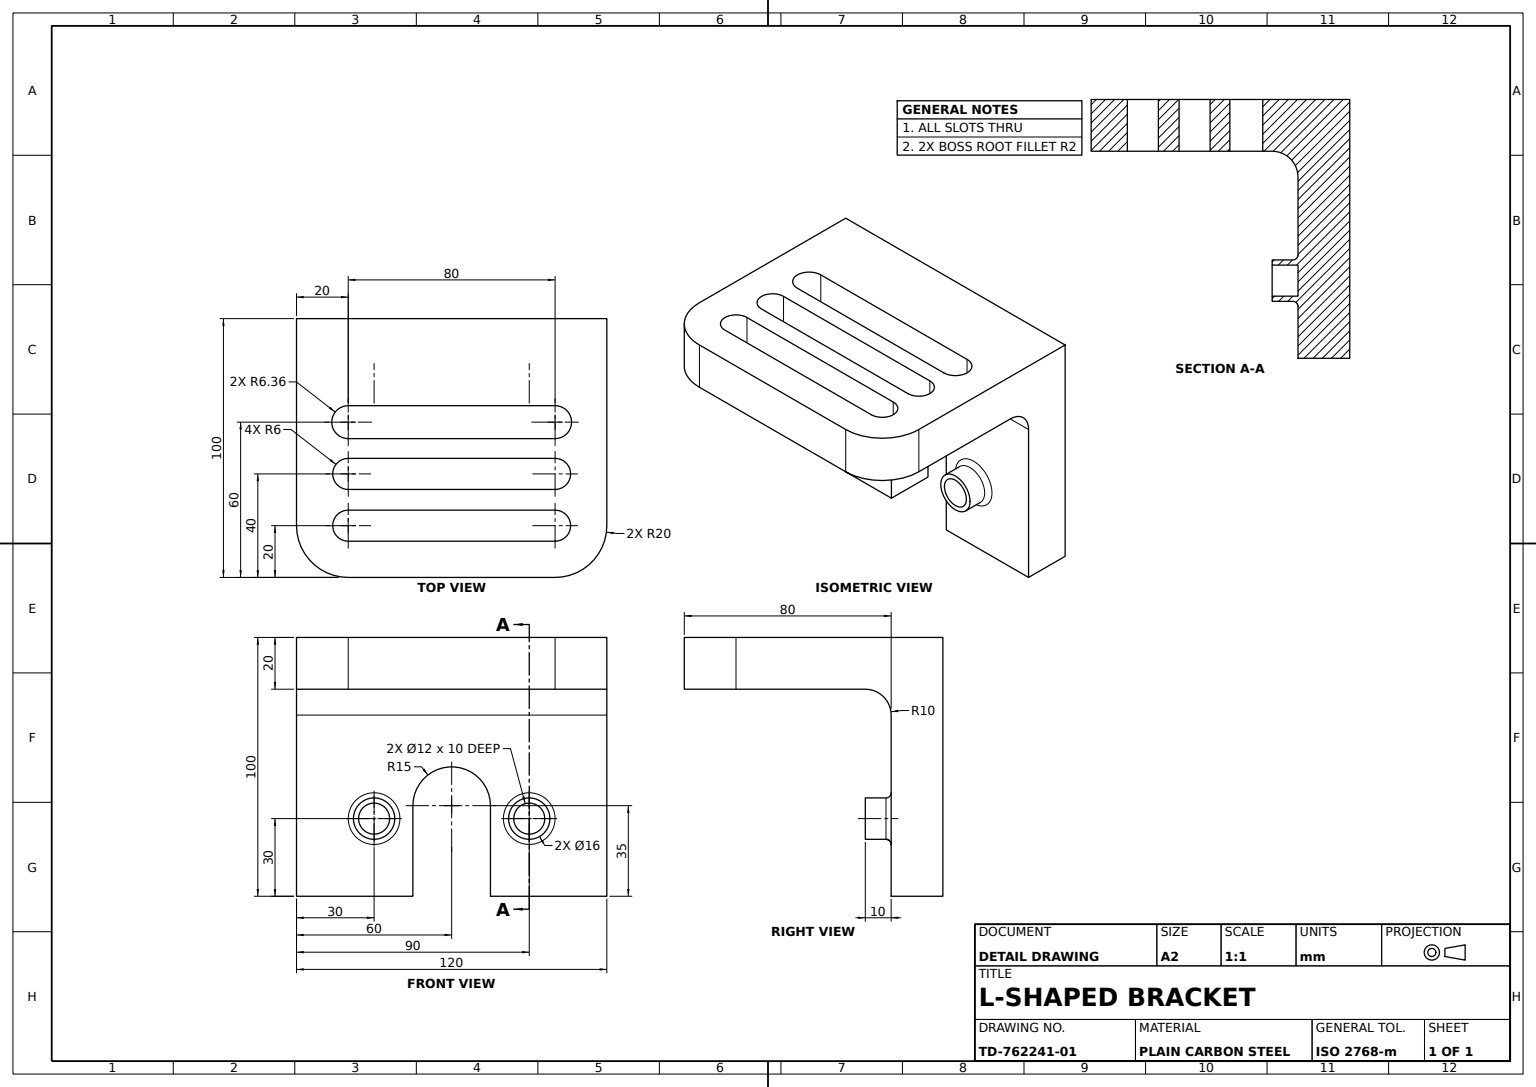
SolidWorks part; units mm, degrees
material "Plain Carbon Steel"
ref_plane "Front Plane" through (0, 0, 0) normal (0, 0, 1) x (1, 0, 0)
ref_plane "Top Plane" through (0, 0, 0) normal (0, 1, 0) x (1, 0, 0)
ref_plane "Right Plane" through (0, 0, 0) normal (1, 0, 0) x (0, 0, -1)
sketch "Back Plate Profile" plane through (0, 0, 0) normal (0, 0, 1) x (1, 0, 0)
  line L0 (0, 0) -> (120, 0)
  line L1 (120, 0) -> (120, 100)
  line L2 (120, 100) -> (0, 100)
  line L3 (0, 100) -> (0, 0)
  dimension "D1" = 120
  dimension "D2" = 100
extrude "Back Plate 120x100x20" add sketch "Back Plate Profile" along normal blind 20
sketch "Top Arm Profile" plane through (0, 0, 20) normal (0, 0, 1) x (1, 0, 0)
  line L0 (120, 100) -> (0, 100) construction
  line L1 (0, 100) -> (120, 100)
  line L2 (0, 100) -> (0, 80)
  line L3 (0, 80) -> (120, 80)
  line L4 (120, 100) -> (120, 80)
  line L5 (0, 100) -> (0, 0) construction
  line L6 (120, 0) -> (120, 100) construction
  dimension "D1" = 20
extrude "Top Arm 80" add sketch "Top Arm Profile" along normal blind 80
sketch "Slot 1 Sketch" plane through (0, 80, 0) normal (0, -1, 0) x (1, 0, 0)
  line L0 (20, 80) -> (100, 80) construction
  line L1 (20, 86) -> (100, 86)
  line L2 (20, 74) -> (100, 74)
  line L4 (0, 100) -> (120, 100) construction
  line L5 (0, 20) -> (120, 20) construction
  arc A0 (20, 86) -> (20, 74) centre (20, 80) ccw
  arc A1 (100, 74) -> (100, 86) centre (100, 80) ccw
  point P2 (60, 80)
  point P9 (60, 100)
  dimension "D1" = 6
  dimension "D2" = 80
  dimension "D3" = 60
extrude "Slot 1 Cut" cut sketch "Slot 1 Sketch" against normal through all
sketch "Slot 2 Sketch" plane through (0, 80, 0) normal (0, -1, 0) x (1, 0, 0)
  line L0 (20, 60) -> (100, 60) construction
  line L1 (20, 66) -> (100, 66)
  line L2 (20, 54) -> (100, 54)
  line L3 (0, 100) -> (120, 100) construction
  arc A0 (20, 66) -> (20, 54) centre (20, 60) ccw
  arc A1 (100, 54) -> (100, 66) centre (100, 60) ccw
  point P2 (60, 60)
  point P9 (60, 100)
  dimension "D2" = 6
  dimension "D1" = 80
  dimension "D3" = 40
extrude "Slot 2 Cut" cut sketch "Slot 2 Sketch" against normal through all
sketch "Slot 3 Sketch" plane through (0, 80, 0) normal (0, -1, 0) x (1, 0, 0)
  line L0 (20, 40) -> (100, 40) construction
  line L1 (20, 46.3649) -> (100, 46.3649)
  line L2 (20, 33.6351) -> (100, 33.6351)
  line L3 (0, 100) -> (120, 100) construction
  arc A0 (20, 46.3649) -> (20, 33.6351) centre (20, 40) ccw
  arc A1 (100, 33.6351) -> (100, 46.3649) centre (100, 40) ccw
  point P2 (60, 40)
  point P9 (60, 100)
  dimension "D3" = 6.3649
  dimension "D1" = 60
  dimension "D2" = 80
extrude "Slot 3 Cut" cut sketch "Slot 3 Sketch" against normal through all
fillet "Arm Root Fillet R10" radius 10 1 edges at (60, 80, 20)
fillet "Arm Corner Round R20" radius 20 2 edges at (120, 90, 100) (0, 90, 100)
sketch "Back Plate Cut Sketch" plane through (0, 0, 20) normal (0, 0, 1) x (1, 0, 0)
  line L0 (60, 0) -> (60, 35) construction
  line L1 (0, 0) -> (120, 0) construction
  line L2 (45, 35) -> (45, 0)
  line L3 (45, 0) -> (75, 0)
  line L4 (75, 0) -> (75, 35)
  line L6 (120, 70) -> (0, 70) construction
  arc A0 (75, 35) -> (45, 35) centre (60, 35) ccw
  dimension "D1" = 30
  dimension "D2" = 35
extrude "Back Plate Cut 30" cut sketch "Back Plate Cut Sketch" against normal through all
sketch "Boss A Sketch" plane through (0, 0, 20) normal (0, 0, 1) x (1, 0, 0)
  line L0 (0, 0) -> (0, 30) construction
  line L1 (0, 70) -> (0, 0) construction
  line L2 (0, 0) -> (30, 0) construction
  line L3 (0, 0) -> (45, 0) construction
  line L4 (30, 0) -> (30, 30) construction
  line L5 (120, 0) -> (120, 70) construction
  circle A0 centre (30, 30) radius 6
  circle A1 centre (30, 30) radius 8
  dimension "D1" = 16
  dimension "D2" = 12
  dimension "D3" = 90
extrude "Mounting Boss A" add sketch "Boss A Sketch" along normal blind 10
sketch "Boss B Sketch" plane through (0, 0, 20) normal (0, 0, 1) x (1, 0, 0)
  line L0 (120, 0) -> (120, 30) construction
  line L1 (120, 0) -> (120, 70) construction
  line L2 (120, 30) -> (90, 30) construction
  circle A0 centre (90, 30) radius 6
  circle A1 centre (90, 30) radius 8
  dimension "D1" = 12
  dimension "D2" = 16
  dimension "D3" = 30
extrude "Mounting Boss B" add sketch "Boss B Sketch" along normal blind 10
fillet "Boss Edge Fillet R2" radius 2 2 edges at (98, 30, 20) (38, 30, 20)
